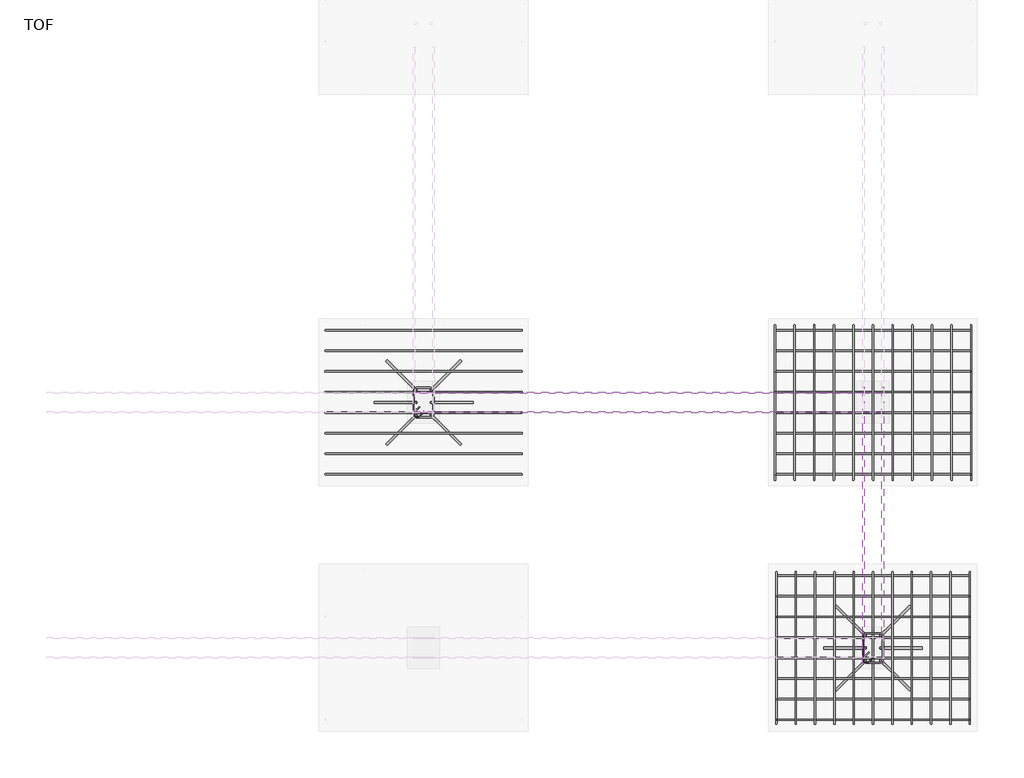
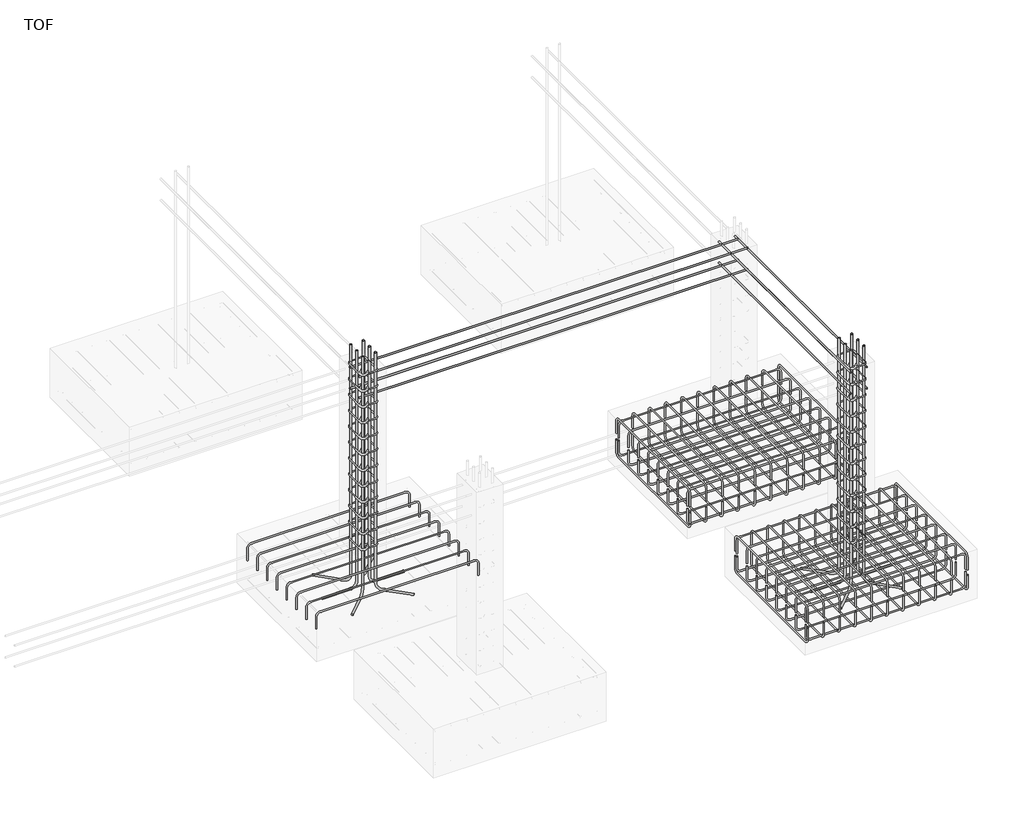
# One storey, part 7 of 10: 31 reinforcing bars.
"""IFC4 building model written with IfcOpenShell, lengths in millimetres."""

from ifc_helpers import new_model, si_unit, point, frame, origin, place, context, project, spatial, polyline, circle_curve, trimmed, segment, composite_curve, source, transform, mapped, element, save
from ifc_brep_helpers import swept_disk

model = new_model("IFC4")

# Units and contexts
model_context = context("Model", 3, world=origin())
ifc_project = project(units=[si_unit("LENGTHUNIT", "METRE", prefix="MILLI")], contexts=[model_context])

# Site, building, storey
site = spatial("IfcSite", under=ifc_project)
building = spatial("IfcBuilding", under=site)
storey = spatial("IfcBuildingStorey", under=building, Name="TOF", Elevation=-1828.8)

# Reinforcing bars
placement = place(None, origin())
reinforcing_bar_shape = source(origin(), model_context, "Body", "SolidModel", [
    swept_disk(composite_curve([segment(polyline([(13565.2782143, -14549.6267376, -2028.8), (13565.2782143, -14549.6267376, -1918.8)]), True, "CONTINUOUS"), segment(trimmed(circle_curve(frame((13565.2782143, -14584.6267376, -1918.8), z_axis=(1.0, 0.0, 0.0), x_axis=(0.0, 35.0, 0.0)), 35.0), [point((13565.2782143, -14549.6267376, -1918.8))], [point((13565.2782143, -14584.6267376, -1883.8))], True, "CARTESIAN"), True, "CONTINUOUS"), segment(polyline([(13565.2782143, -14584.6267376, -1883.8), (13565.2782143, -15604.6267376, -1883.8)]), True, "CONTINUOUS"), segment(trimmed(circle_curve(frame((13565.2782143, -15604.6267376, -1918.8), z_axis=(1.0, 0.0, 0.0), x_axis=(0.0, 0.0, 35.0)), 35.0), [point((13565.2782143, -15604.6267376, -1883.8))], [point((13565.2782143, -15639.6267376, -1918.8))], True, "CARTESIAN"), True, "CONTINUOUS"), segment(polyline([(13565.2782143, -15639.6267376, -1918.8), (13565.2782143, -15639.6267376, -2028.8)]), True, "CONTINUOUS")], self_intersect=False), 5.0),
])
element("IfcReinforcingBar", 1, at=placement, inside=storey, context=model_context, shape_type="MappedRepresentation", body=[
    mapped(reinforcing_bar_shape, transform((0.0, 0.0, 0.0), x_axis=(1.0, 0.0, 0.0), y_axis=(0.0, 1.0, 0.0), z_axis=(0.0, 0.0, 1.0))),
    mapped(reinforcing_bar_shape, transform((-139.0, 0.0, 0.0), x_axis=(1.0, 0.0, 0.0), y_axis=(0.0, 1.0, 0.0), z_axis=(0.0, 0.0, 1.0))),
    mapped(reinforcing_bar_shape, transform((-278.0, 0.0, 0.0), x_axis=(1.0, 0.0, 0.0), y_axis=(0.0, 1.0, 0.0), z_axis=(0.0, 0.0, 1.0))),
    mapped(reinforcing_bar_shape, transform((-417.0, 0.0, 0.0), x_axis=(1.0, 0.0, 0.0), y_axis=(0.0, 1.0, 0.0), z_axis=(0.0, 0.0, 1.0))),
    mapped(reinforcing_bar_shape, transform((-556.0, 0.0, 0.0), x_axis=(1.0, 0.0, 0.0), y_axis=(0.0, 1.0, 0.0), z_axis=(0.0, 0.0, 1.0))),
    mapped(reinforcing_bar_shape, transform((-695.0, 0.0, 0.0), x_axis=(1.0, 0.0, 0.0), y_axis=(0.0, 1.0, 0.0), z_axis=(0.0, 0.0, 1.0))),
    mapped(reinforcing_bar_shape, transform((-834.0, 0.0, 0.0), x_axis=(1.0, 0.0, 0.0), y_axis=(0.0, 1.0, 0.0), z_axis=(0.0, 0.0, 1.0))),
    mapped(reinforcing_bar_shape, transform((-973.0, 0.0, 0.0), x_axis=(1.0, 0.0, 0.0), y_axis=(0.0, 1.0, 0.0), z_axis=(0.0, 0.0, 1.0))),
    mapped(reinforcing_bar_shape, transform((-1112.0, 0.0, 0.0), x_axis=(1.0, 0.0, 0.0), y_axis=(0.0, 1.0, 0.0), z_axis=(0.0, 0.0, 1.0))),
    mapped(reinforcing_bar_shape, transform((-1251.0, 0.0, 0.0), x_axis=(1.0, 0.0, 0.0), y_axis=(0.0, 1.0, 0.0), z_axis=(0.0, 0.0, 1.0))),
    mapped(reinforcing_bar_shape, transform((-1390.0, 0.0, 0.0), x_axis=(1.0, 0.0, 0.0), y_axis=(0.0, 1.0, 0.0), z_axis=(0.0, 0.0, 1.0))),
])
reinforcing_bar_2_shape = source(origin(), model_context, "Body", "SolidModel", [
    swept_disk(composite_curve([segment(polyline([(13565.2782143, -15639.6267376, -2077.5233378), (13565.2782143, -15639.6267376, -2187.5233378)]), True, "CONTINUOUS"), segment(trimmed(circle_curve(frame((13565.2782143, -15604.6267376, -2187.5233378), z_axis=(1.0, 0.0, 0.0), x_axis=(0.0, -35.0, 0.0)), 35.0), [point((13565.2782143, -15639.6267376, -2187.5233378))], [point((13565.2782143, -15604.6267376, -2222.5233378))], True, "CARTESIAN"), True, "CONTINUOUS"), segment(polyline([(13565.2782143, -15604.6267376, -2222.5233378), (13565.2782143, -14584.6267376, -2222.5233378)]), True, "CONTINUOUS"), segment(trimmed(circle_curve(frame((13565.2782143, -14584.6267376, -2187.5233378), z_axis=(1.0, 0.0, 0.0), x_axis=(0.0, 0.0, -35.0)), 35.0), [point((13565.2782143, -14584.6267376, -2222.5233378))], [point((13565.2782143, -14549.6267376, -2187.5233378))], True, "CARTESIAN"), True, "CONTINUOUS"), segment(polyline([(13565.2782143, -14549.6267376, -2187.5233378), (13565.2782143, -14549.6267376, -2077.5233378)]), True, "CONTINUOUS")], self_intersect=False), 5.0),
])
element("IfcReinforcingBar", 2, at=placement, inside=storey, context=model_context, shape_type="MappedRepresentation", body=[
    mapped(reinforcing_bar_2_shape, transform((0.0, 0.0, 0.0), x_axis=(1.0, 0.0, 0.0), y_axis=(0.0, 1.0, 0.0), z_axis=(0.0, 0.0, 1.0))),
    mapped(reinforcing_bar_2_shape, transform((-139.0, 0.0, 0.0), x_axis=(1.0, 0.0, 0.0), y_axis=(0.0, 1.0, 0.0), z_axis=(0.0, 0.0, 1.0))),
    mapped(reinforcing_bar_2_shape, transform((-278.0, 0.0, 0.0), x_axis=(1.0, 0.0, 0.0), y_axis=(0.0, 1.0, 0.0), z_axis=(0.0, 0.0, 1.0))),
    mapped(reinforcing_bar_2_shape, transform((-417.0, 0.0, 0.0), x_axis=(1.0, 0.0, 0.0), y_axis=(0.0, 1.0, 0.0), z_axis=(0.0, 0.0, 1.0))),
    mapped(reinforcing_bar_2_shape, transform((-556.0, 0.0, 0.0), x_axis=(1.0, 0.0, 0.0), y_axis=(0.0, 1.0, 0.0), z_axis=(0.0, 0.0, 1.0))),
    mapped(reinforcing_bar_2_shape, transform((-695.0, 0.0, 0.0), x_axis=(1.0, 0.0, 0.0), y_axis=(0.0, 1.0, 0.0), z_axis=(0.0, 0.0, 1.0))),
    mapped(reinforcing_bar_2_shape, transform((-834.0, 0.0, 0.0), x_axis=(1.0, 0.0, 0.0), y_axis=(0.0, 1.0, 0.0), z_axis=(0.0, 0.0, 1.0))),
    mapped(reinforcing_bar_2_shape, transform((-973.0, 0.0, 0.0), x_axis=(1.0, 0.0, 0.0), y_axis=(0.0, 1.0, 0.0), z_axis=(0.0, 0.0, 1.0))),
    mapped(reinforcing_bar_2_shape, transform((-1112.0, 0.0, 0.0), x_axis=(1.0, 0.0, 0.0), y_axis=(0.0, 1.0, 0.0), z_axis=(0.0, 0.0, 1.0))),
    mapped(reinforcing_bar_2_shape, transform((-1251.0, 0.0, 0.0), x_axis=(1.0, 0.0, 0.0), y_axis=(0.0, 1.0, 0.0), z_axis=(0.0, 0.0, 1.0))),
    mapped(reinforcing_bar_2_shape, transform((-1390.0, 0.0, 0.0), x_axis=(1.0, 0.0, 0.0), y_axis=(0.0, 1.0, 0.0), z_axis=(0.0, 0.0, 1.0))),
])
reinforcing_bar_3_shape = source(origin(), model_context, "Body", "SolidModel", [
    swept_disk(composite_curve([segment(polyline([(13565.2782143, -14574.6861459, -2066.1776706), (13565.2782143, -14574.6861459, -2176.1776706)]), True, "CONTINUOUS"), segment(trimmed(circle_curve(frame((13530.2782143, -14574.6861459, -2176.1776706), z_axis=(0.0, 1.0, 0.0), x_axis=(35.0, 0.0, 0.0)), 35.0), [point((13565.2782143, -14574.6861459, -2176.1776706))], [point((13530.2782143, -14574.6861459, -2211.1776706))], True, "CARTESIAN"), True, "CONTINUOUS"), segment(polyline([(13530.2782143, -14574.6861459, -2211.1776706), (12210.2782143, -14574.6861459, -2211.1776706)]), True, "CONTINUOUS"), segment(trimmed(circle_curve(frame((12210.2782143, -14574.6861459, -2176.1776706), z_axis=(0.0, 1.0, 0.0), x_axis=(0.0, 0.0, -35.0)), 35.0), [point((12210.2782143, -14574.6861459, -2211.1776706))], [point((12175.2782143, -14574.6861459, -2176.1776706))], True, "CARTESIAN"), True, "CONTINUOUS"), segment(polyline([(12175.2782143, -14574.6861459, -2176.1776706), (12175.2782143, -14574.6861459, -2066.1776706)]), True, "CONTINUOUS")], self_intersect=False), 5.0),
])
element("IfcReinforcingBar", 3, at=placement, inside=storey, context=model_context, shape_type="MappedRepresentation", body=[
    mapped(reinforcing_bar_3_shape, transform((0.0, 0.0, 0.0), x_axis=(1.0, 0.0, 0.0), y_axis=(0.0, 1.0, 0.0), z_axis=(0.0, 0.0, 1.0))),
    mapped(reinforcing_bar_3_shape, transform((0.0, -148.0321606, 0.0), x_axis=(1.0, 0.0, 0.0), y_axis=(0.0, 1.0, 0.0), z_axis=(0.0, 0.0, 1.0))),
    mapped(reinforcing_bar_3_shape, transform((0.0, -296.0643211, 0.0), x_axis=(1.0, 0.0, 0.0), y_axis=(0.0, 1.0, 0.0), z_axis=(0.0, 0.0, 1.0))),
    mapped(reinforcing_bar_3_shape, transform((0.0, -444.0964817, 0.0), x_axis=(1.0, 0.0, 0.0), y_axis=(0.0, 1.0, 0.0), z_axis=(0.0, 0.0, 1.0))),
    mapped(reinforcing_bar_3_shape, transform((0.0, -592.1286423, 0.0), x_axis=(1.0, 0.0, 0.0), y_axis=(0.0, 1.0, 0.0), z_axis=(0.0, 0.0, 1.0))),
    mapped(reinforcing_bar_3_shape, transform((0.0, -740.1608029, 0.0), x_axis=(1.0, 0.0, 0.0), y_axis=(0.0, 1.0, 0.0), z_axis=(0.0, 0.0, 1.0))),
    mapped(reinforcing_bar_3_shape, transform((0.0, -888.1929634, 0.0), x_axis=(1.0, 0.0, 0.0), y_axis=(0.0, 1.0, 0.0), z_axis=(0.0, 0.0, 1.0))),
    mapped(reinforcing_bar_3_shape, transform((0.0, -1036.225124, 0.0), x_axis=(1.0, 0.0, 0.0), y_axis=(0.0, 1.0, 0.0), z_axis=(0.0, 0.0, 1.0))),
])
reinforcing_bar_4_shape = source(origin(), model_context, "Body", "SolidModel", [
    swept_disk(composite_curve([segment(polyline([(13565.2782143, -15610.9112699, -2039.256778), (13565.2782143, -15610.9112699, -1929.256778)]), True, "CONTINUOUS"), segment(trimmed(circle_curve(frame((13530.2782143, -15610.9112699, -1929.256778), z_axis=(0.0, -1.0, 0.0), x_axis=(35.0, 0.0, 0.0)), 35.0), [point((13565.2782143, -15610.9112699, -1929.256778))], [point((13530.2782143, -15610.9112699, -1894.256778))], True, "CARTESIAN"), True, "CONTINUOUS"), segment(polyline([(13530.2782143, -15610.9112699, -1894.256778), (12210.2782143, -15610.9112699, -1894.256778)]), True, "CONTINUOUS"), segment(trimmed(circle_curve(frame((12210.2782143, -15610.9112699, -1929.256778), z_axis=(0.0, -1.0, 0.0), x_axis=(0.0, 0.0, 35.0)), 35.0), [point((12210.2782143, -15610.9112699, -1894.256778))], [point((12175.2782143, -15610.9112699, -1929.256778))], True, "CARTESIAN"), True, "CONTINUOUS"), segment(polyline([(12175.2782143, -15610.9112699, -1929.256778), (12175.2782143, -15610.9112699, -2039.256778)]), True, "CONTINUOUS")], self_intersect=False), 5.0),
])
element("IfcReinforcingBar", 4, at=placement, inside=storey, context=model_context, shape_type="MappedRepresentation", body=[
    mapped(reinforcing_bar_4_shape, transform((0.0, 0.0, 0.0), x_axis=(1.0, 0.0, 0.0), y_axis=(0.0, 1.0, 0.0), z_axis=(0.0, 0.0, 1.0))),
    mapped(reinforcing_bar_4_shape, transform((0.0, 148.0321606, 0.0), x_axis=(1.0, 0.0, 0.0), y_axis=(0.0, 1.0, 0.0), z_axis=(0.0, 0.0, 1.0))),
    mapped(reinforcing_bar_4_shape, transform((0.0, 296.0643211, 0.0), x_axis=(1.0, 0.0, 0.0), y_axis=(0.0, 1.0, 0.0), z_axis=(0.0, 0.0, 1.0))),
    mapped(reinforcing_bar_4_shape, transform((0.0, 444.0964817, 0.0), x_axis=(1.0, 0.0, 0.0), y_axis=(0.0, 1.0, 0.0), z_axis=(0.0, 0.0, 1.0))),
    mapped(reinforcing_bar_4_shape, transform((0.0, 592.1286423, 0.0), x_axis=(1.0, 0.0, 0.0), y_axis=(0.0, 1.0, 0.0), z_axis=(0.0, 0.0, 1.0))),
    mapped(reinforcing_bar_4_shape, transform((0.0, 740.1608029, 0.0), x_axis=(1.0, 0.0, 0.0), y_axis=(0.0, 1.0, 0.0), z_axis=(0.0, 0.0, 1.0))),
    mapped(reinforcing_bar_4_shape, transform((0.0, 888.1929634, 0.0), x_axis=(1.0, 0.0, 0.0), y_axis=(0.0, 1.0, 0.0), z_axis=(0.0, 0.0, 1.0))),
    mapped(reinforcing_bar_4_shape, transform((0.0, 1036.225124, 0.0), x_axis=(1.0, 0.0, 0.0), y_axis=(0.0, 1.0, 0.0), z_axis=(0.0, 0.0, 1.0))),
])
reinforcing_bar_5_shape = source(origin(), model_context, "Body", "SolidModel", [
    swept_disk(composite_curve([segment(polyline([(10345.2782143, -13845.9112699, -2039.256778), (10345.2782143, -13845.9112699, -1929.256778)]), True, "CONTINUOUS"), segment(trimmed(circle_curve(frame((10310.2782143, -13845.9112699, -1929.256778), z_axis=(0.0, -1.0, 0.0), x_axis=(35.0, 0.0, 0.0)), 35.0), [point((10345.2782143, -13845.9112699, -1929.256778))], [point((10310.2782143, -13845.9112699, -1894.256778))], True, "CARTESIAN"), True, "CONTINUOUS"), segment(polyline([(10310.2782143, -13845.9112699, -1894.256778), (8970.2782143, -13845.9112699, -1894.256778)]), True, "CONTINUOUS"), segment(trimmed(circle_curve(frame((8970.2782143, -13845.9112699, -1929.256778), z_axis=(0.0, -1.0, 0.0), x_axis=(0.0, 0.0, 35.0)), 35.0), [point((8970.2782143, -13845.9112699, -1894.256778))], [point((8935.2782143, -13845.9112699, -1929.256778))], True, "CARTESIAN"), True, "CONTINUOUS"), segment(polyline([(8935.2782143, -13845.9112699, -1929.256778), (8935.2782143, -13845.9112699, -2039.256778)]), True, "CONTINUOUS")], self_intersect=False), 5.0),
])
element("IfcReinforcingBar", 5, at=placement, inside=storey, context=model_context, shape_type="MappedRepresentation", body=[
    mapped(reinforcing_bar_5_shape, transform((0.0, 0.0, 0.0), x_axis=(1.0, 0.0, 0.0), y_axis=(0.0, 1.0, 0.0), z_axis=(0.0, 0.0, 1.0))),
    mapped(reinforcing_bar_5_shape, transform((0.0, 148.0321606, 0.0), x_axis=(1.0, 0.0, 0.0), y_axis=(0.0, 1.0, 0.0), z_axis=(0.0, 0.0, 1.0))),
    mapped(reinforcing_bar_5_shape, transform((0.0, 296.0643211, 0.0), x_axis=(1.0, 0.0, 0.0), y_axis=(0.0, 1.0, 0.0), z_axis=(0.0, 0.0, 1.0))),
    mapped(reinforcing_bar_5_shape, transform((0.0, 444.0964817, 0.0), x_axis=(1.0, 0.0, 0.0), y_axis=(0.0, 1.0, 0.0), z_axis=(0.0, 0.0, 1.0))),
    mapped(reinforcing_bar_5_shape, transform((0.0, 592.1286423, 0.0), x_axis=(1.0, 0.0, 0.0), y_axis=(0.0, 1.0, 0.0), z_axis=(0.0, 0.0, 1.0))),
    mapped(reinforcing_bar_5_shape, transform((0.0, 740.1608029, 0.0), x_axis=(1.0, 0.0, 0.0), y_axis=(0.0, 1.0, 0.0), z_axis=(0.0, 0.0, 1.0))),
    mapped(reinforcing_bar_5_shape, transform((0.0, 888.1929634, 0.0), x_axis=(1.0, 0.0, 0.0), y_axis=(0.0, 1.0, 0.0), z_axis=(0.0, 0.0, 1.0))),
    mapped(reinforcing_bar_5_shape, transform((0.0, 1036.225124, 0.0), x_axis=(1.0, 0.0, 0.0), y_axis=(0.0, 1.0, 0.0), z_axis=(0.0, 0.0, 1.0))),
])
reinforcing_bar_6_shape = source(origin(), model_context, "Body", "SolidModel", [
    swept_disk(composite_curve([segment(polyline([(13575.2782143, -12774.6267376, -2018.8), (13575.2782143, -12774.6267376, -1908.8)]), True, "CONTINUOUS"), segment(trimmed(circle_curve(frame((13575.2782143, -12809.6267376, -1908.8), z_axis=(1.0, 0.0, 0.0), x_axis=(0.0, 35.0, 0.0)), 35.0), [point((13575.2782143, -12774.6267376, -1908.8))], [point((13575.2782143, -12809.6267376, -1873.8))], True, "CARTESIAN"), True, "CONTINUOUS"), segment(polyline([(13575.2782143, -12809.6267376, -1873.8), (13575.2782143, -13849.6267376, -1873.8)]), True, "CONTINUOUS"), segment(trimmed(circle_curve(frame((13575.2782143, -13849.6267376, -1908.8), z_axis=(1.0, 0.0, 0.0), x_axis=(0.0, 0.0, 35.0)), 35.0), [point((13575.2782143, -13849.6267376, -1873.8))], [point((13575.2782143, -13884.6267376, -1908.8))], True, "CARTESIAN"), True, "CONTINUOUS"), segment(polyline([(13575.2782143, -13884.6267376, -1908.8), (13575.2782143, -13884.6267376, -2018.8)]), True, "CONTINUOUS")], self_intersect=False), 5.0),
])
element("IfcReinforcingBar", 6, at=placement, inside=storey, context=model_context, shape_type="MappedRepresentation", body=[
    mapped(reinforcing_bar_6_shape, transform((0.0, 0.0, 0.0), x_axis=(1.0, 0.0, 0.0), y_axis=(0.0, 1.0, 0.0), z_axis=(0.0, 0.0, 1.0))),
    mapped(reinforcing_bar_6_shape, transform((-141.0, 0.0, 0.0), x_axis=(1.0, 0.0, 0.0), y_axis=(0.0, 1.0, 0.0), z_axis=(0.0, 0.0, 1.0))),
    mapped(reinforcing_bar_6_shape, transform((-282.0, 0.0, 0.0), x_axis=(1.0, 0.0, 0.0), y_axis=(0.0, 1.0, 0.0), z_axis=(0.0, 0.0, 1.0))),
    mapped(reinforcing_bar_6_shape, transform((-423.0, 0.0, 0.0), x_axis=(1.0, 0.0, 0.0), y_axis=(0.0, 1.0, 0.0), z_axis=(0.0, 0.0, 1.0))),
    mapped(reinforcing_bar_6_shape, transform((-564.0, 0.0, 0.0), x_axis=(1.0, 0.0, 0.0), y_axis=(0.0, 1.0, 0.0), z_axis=(0.0, 0.0, 1.0))),
    mapped(reinforcing_bar_6_shape, transform((-705.0, 0.0, 0.0), x_axis=(1.0, 0.0, 0.0), y_axis=(0.0, 1.0, 0.0), z_axis=(0.0, 0.0, 1.0))),
    mapped(reinforcing_bar_6_shape, transform((-846.0, 0.0, 0.0), x_axis=(1.0, 0.0, 0.0), y_axis=(0.0, 1.0, 0.0), z_axis=(0.0, 0.0, 1.0))),
    mapped(reinforcing_bar_6_shape, transform((-987.0, 0.0, 0.0), x_axis=(1.0, 0.0, 0.0), y_axis=(0.0, 1.0, 0.0), z_axis=(0.0, 0.0, 1.0))),
    mapped(reinforcing_bar_6_shape, transform((-1128.0, 0.0, 0.0), x_axis=(1.0, 0.0, 0.0), y_axis=(0.0, 1.0, 0.0), z_axis=(0.0, 0.0, 1.0))),
    mapped(reinforcing_bar_6_shape, transform((-1269.0, 0.0, 0.0), x_axis=(1.0, 0.0, 0.0), y_axis=(0.0, 1.0, 0.0), z_axis=(0.0, 0.0, 1.0))),
    mapped(reinforcing_bar_6_shape, transform((-1410.0, 0.0, 0.0), x_axis=(1.0, 0.0, 0.0), y_axis=(0.0, 1.0, 0.0), z_axis=(0.0, 0.0, 1.0))),
])
reinforcing_bar_7_shape = source(origin(), model_context, "Body", "SolidModel", [
    swept_disk(composite_curve([segment(polyline([(13575.2782143, -13884.6267376, -2077.5233378), (13575.2782143, -13884.6267376, -2187.5233378)]), True, "CONTINUOUS"), segment(trimmed(circle_curve(frame((13575.2782143, -13849.6267376, -2187.5233378), z_axis=(1.0, 0.0, 0.0), x_axis=(0.0, -35.0, 0.0)), 35.0), [point((13575.2782143, -13884.6267376, -2187.5233378))], [point((13575.2782143, -13849.6267376, -2222.5233378))], True, "CARTESIAN"), True, "CONTINUOUS"), segment(polyline([(13575.2782143, -13849.6267376, -2222.5233378), (13575.2782143, -12809.6267376, -2222.5233378)]), True, "CONTINUOUS"), segment(trimmed(circle_curve(frame((13575.2782143, -12809.6267376, -2187.5233378), z_axis=(1.0, 0.0, 0.0), x_axis=(0.0, 0.0, -35.0)), 35.0), [point((13575.2782143, -12809.6267376, -2222.5233378))], [point((13575.2782143, -12774.6267376, -2187.5233378))], True, "CARTESIAN"), True, "CONTINUOUS"), segment(polyline([(13575.2782143, -12774.6267376, -2187.5233378), (13575.2782143, -12774.6267376, -2077.5233378)]), True, "CONTINUOUS")], self_intersect=False), 5.0),
])
element("IfcReinforcingBar", 7, at=placement, inside=storey, context=model_context, shape_type="MappedRepresentation", body=[
    mapped(reinforcing_bar_7_shape, transform((0.0, 0.0, 0.0), x_axis=(1.0, 0.0, 0.0), y_axis=(0.0, 1.0, 0.0), z_axis=(0.0, 0.0, 1.0))),
    mapped(reinforcing_bar_7_shape, transform((-141.0, 0.0, 0.0), x_axis=(1.0, 0.0, 0.0), y_axis=(0.0, 1.0, 0.0), z_axis=(0.0, 0.0, 1.0))),
    mapped(reinforcing_bar_7_shape, transform((-282.0, 0.0, 0.0), x_axis=(1.0, 0.0, 0.0), y_axis=(0.0, 1.0, 0.0), z_axis=(0.0, 0.0, 1.0))),
    mapped(reinforcing_bar_7_shape, transform((-423.0, 0.0, 0.0), x_axis=(1.0, 0.0, 0.0), y_axis=(0.0, 1.0, 0.0), z_axis=(0.0, 0.0, 1.0))),
    mapped(reinforcing_bar_7_shape, transform((-564.0, 0.0, 0.0), x_axis=(1.0, 0.0, 0.0), y_axis=(0.0, 1.0, 0.0), z_axis=(0.0, 0.0, 1.0))),
    mapped(reinforcing_bar_7_shape, transform((-705.0, 0.0, 0.0), x_axis=(1.0, 0.0, 0.0), y_axis=(0.0, 1.0, 0.0), z_axis=(0.0, 0.0, 1.0))),
    mapped(reinforcing_bar_7_shape, transform((-846.0, 0.0, 0.0), x_axis=(1.0, 0.0, 0.0), y_axis=(0.0, 1.0, 0.0), z_axis=(0.0, 0.0, 1.0))),
    mapped(reinforcing_bar_7_shape, transform((-987.0, 0.0, 0.0), x_axis=(1.0, 0.0, 0.0), y_axis=(0.0, 1.0, 0.0), z_axis=(0.0, 0.0, 1.0))),
    mapped(reinforcing_bar_7_shape, transform((-1128.0, 0.0, 0.0), x_axis=(1.0, 0.0, 0.0), y_axis=(0.0, 1.0, 0.0), z_axis=(0.0, 0.0, 1.0))),
    mapped(reinforcing_bar_7_shape, transform((-1269.0, 0.0, 0.0), x_axis=(1.0, 0.0, 0.0), y_axis=(0.0, 1.0, 0.0), z_axis=(0.0, 0.0, 1.0))),
    mapped(reinforcing_bar_7_shape, transform((-1410.0, 0.0, 0.0), x_axis=(1.0, 0.0, 0.0), y_axis=(0.0, 1.0, 0.0), z_axis=(0.0, 0.0, 1.0))),
])
reinforcing_bar_8_shape = source(origin(), model_context, "Body", "SolidModel", [
    swept_disk(composite_curve([segment(polyline([(13575.2782143, -12809.6861459, -2066.1776706), (13575.2782143, -12809.6861459, -2176.1776706)]), True, "CONTINUOUS"), segment(trimmed(circle_curve(frame((13540.2782143, -12809.6861459, -2176.1776706), z_axis=(0.0, 1.0, 0.0), x_axis=(35.0, 0.0, 0.0)), 35.0), [point((13575.2782143, -12809.6861459, -2176.1776706))], [point((13540.2782143, -12809.6861459, -2211.1776706))], True, "CARTESIAN"), True, "CONTINUOUS"), segment(polyline([(13540.2782143, -12809.6861459, -2211.1776706), (12200.2782143, -12809.6861459, -2211.1776706)]), True, "CONTINUOUS"), segment(trimmed(circle_curve(frame((12200.2782143, -12809.6861459, -2176.1776706), z_axis=(0.0, 1.0, 0.0), x_axis=(0.0, 0.0, -35.0)), 35.0), [point((12200.2782143, -12809.6861459, -2211.1776706))], [point((12165.2782143, -12809.6861459, -2176.1776706))], True, "CARTESIAN"), True, "CONTINUOUS"), segment(polyline([(12165.2782143, -12809.6861459, -2176.1776706), (12165.2782143, -12809.6861459, -2066.1776706)]), True, "CONTINUOUS")], self_intersect=False), 5.0),
])
element("IfcReinforcingBar", 8, at=placement, inside=storey, context=model_context, shape_type="MappedRepresentation", body=[
    mapped(reinforcing_bar_8_shape, transform((0.0, 0.0, 0.0), x_axis=(1.0, 0.0, 0.0), y_axis=(0.0, 1.0, 0.0), z_axis=(0.0, 0.0, 1.0))),
    mapped(reinforcing_bar_8_shape, transform((0.0, -148.0321606, 0.0), x_axis=(1.0, 0.0, 0.0), y_axis=(0.0, 1.0, 0.0), z_axis=(0.0, 0.0, 1.0))),
    mapped(reinforcing_bar_8_shape, transform((0.0, -296.0643211, 0.0), x_axis=(1.0, 0.0, 0.0), y_axis=(0.0, 1.0, 0.0), z_axis=(0.0, 0.0, 1.0))),
    mapped(reinforcing_bar_8_shape, transform((0.0, -444.0964817, 0.0), x_axis=(1.0, 0.0, 0.0), y_axis=(0.0, 1.0, 0.0), z_axis=(0.0, 0.0, 1.0))),
    mapped(reinforcing_bar_8_shape, transform((0.0, -592.1286423, 0.0), x_axis=(1.0, 0.0, 0.0), y_axis=(0.0, 1.0, 0.0), z_axis=(0.0, 0.0, 1.0))),
    mapped(reinforcing_bar_8_shape, transform((0.0, -740.1608029, 0.0), x_axis=(1.0, 0.0, 0.0), y_axis=(0.0, 1.0, 0.0), z_axis=(0.0, 0.0, 1.0))),
    mapped(reinforcing_bar_8_shape, transform((0.0, -888.1929634, 0.0), x_axis=(1.0, 0.0, 0.0), y_axis=(0.0, 1.0, 0.0), z_axis=(0.0, 0.0, 1.0))),
    mapped(reinforcing_bar_8_shape, transform((0.0, -1036.225124, 0.0), x_axis=(1.0, 0.0, 0.0), y_axis=(0.0, 1.0, 0.0), z_axis=(0.0, 0.0, 1.0))),
])
reinforcing_bar_9_shape = source(origin(), model_context, "Body", "SolidModel", [
    swept_disk(composite_curve([segment(polyline([(13575.2782143, -13845.9112699, -2039.256778), (13575.2782143, -13845.9112699, -1929.256778)]), True, "CONTINUOUS"), segment(trimmed(circle_curve(frame((13540.2782143, -13845.9112699, -1929.256778), z_axis=(0.0, -1.0, 0.0), x_axis=(35.0, 0.0, 0.0)), 35.0), [point((13575.2782143, -13845.9112699, -1929.256778))], [point((13540.2782143, -13845.9112699, -1894.256778))], True, "CARTESIAN"), True, "CONTINUOUS"), segment(polyline([(13540.2782143, -13845.9112699, -1894.256778), (12200.2782143, -13845.9112699, -1894.256778)]), True, "CONTINUOUS"), segment(trimmed(circle_curve(frame((12200.2782143, -13845.9112699, -1929.256778), z_axis=(0.0, -1.0, 0.0), x_axis=(0.0, 0.0, 35.0)), 35.0), [point((12200.2782143, -13845.9112699, -1894.256778))], [point((12165.2782143, -13845.9112699, -1929.256778))], True, "CARTESIAN"), True, "CONTINUOUS"), segment(polyline([(12165.2782143, -13845.9112699, -1929.256778), (12165.2782143, -13845.9112699, -2039.256778)]), True, "CONTINUOUS")], self_intersect=False), 5.0),
])
element("IfcReinforcingBar", 9, at=placement, inside=storey, context=model_context, shape_type="MappedRepresentation", body=[
    mapped(reinforcing_bar_9_shape, transform((0.0, 0.0, 0.0), x_axis=(1.0, 0.0, 0.0), y_axis=(0.0, 1.0, 0.0), z_axis=(0.0, 0.0, 1.0))),
    mapped(reinforcing_bar_9_shape, transform((0.0, 148.0321606, 0.0), x_axis=(1.0, 0.0, 0.0), y_axis=(0.0, 1.0, 0.0), z_axis=(0.0, 0.0, 1.0))),
    mapped(reinforcing_bar_9_shape, transform((0.0, 296.0643211, 0.0), x_axis=(1.0, 0.0, 0.0), y_axis=(0.0, 1.0, 0.0), z_axis=(0.0, 0.0, 1.0))),
    mapped(reinforcing_bar_9_shape, transform((0.0, 444.0964817, 0.0), x_axis=(1.0, 0.0, 0.0), y_axis=(0.0, 1.0, 0.0), z_axis=(0.0, 0.0, 1.0))),
    mapped(reinforcing_bar_9_shape, transform((0.0, 592.1286423, 0.0), x_axis=(1.0, 0.0, 0.0), y_axis=(0.0, 1.0, 0.0), z_axis=(0.0, 0.0, 1.0))),
    mapped(reinforcing_bar_9_shape, transform((0.0, 740.1608029, 0.0), x_axis=(1.0, 0.0, 0.0), y_axis=(0.0, 1.0, 0.0), z_axis=(0.0, 0.0, 1.0))),
    mapped(reinforcing_bar_9_shape, transform((0.0, 888.1929634, 0.0), x_axis=(1.0, 0.0, 0.0), y_axis=(0.0, 1.0, 0.0), z_axis=(0.0, 0.0, 1.0))),
    mapped(reinforcing_bar_9_shape, transform((0.0, 1036.225124, 0.0), x_axis=(1.0, 0.0, 0.0), y_axis=(0.0, 1.0, 0.0), z_axis=(0.0, 0.0, 1.0))),
])
reinforcing_bar_10_shape = source(origin(), model_context, "Body", "SolidModel", [
    swept_disk(composite_curve([segment(polyline([(12840.248777, -15125.7150493, -1784.8), (12806.3076515, -15159.6561748, -1784.8)]), True, "CONTINUOUS"), segment(trimmed(circle_curve(frame((12823.2782143, -15176.6267376, -1784.8), z_axis=(0.0, 0.0, 1.0), x_axis=(-16.970562800001062, 16.970562799999243, 0.0)), 24.0), [point((12806.3076515, -15159.6561748, -1784.8))], [point((12823.2782143, -15200.6267376, -1784.8))], True, "CARTESIAN"), True, "CONTINUOUS"), segment(polyline([(12823.2782143, -15200.6267376, -1784.8), (12917.2782143, -15200.6267376, -1784.8)]), True, "CONTINUOUS"), segment(trimmed(circle_curve(frame((12917.2782143, -15176.6267376, -1784.8), z_axis=(0.0, 0.0, 1.0), x_axis=(0.0, -24.0, 0.0)), 24.0), [point((12917.2782143, -15200.6267376, -1784.8))], [point((12941.2782143, -15176.6267376, -1784.8))], True, "CARTESIAN"), True, "CONTINUOUS"), segment(polyline([(12941.2782143, -15176.6267376, -1784.8), (12941.2782143, -15012.6267376, -1784.8)]), True, "CONTINUOUS"), segment(trimmed(circle_curve(frame((12917.3162115, -15012.6267376, -1786.149972), z_axis=(-0.05624883273897078, 0.0, 0.9984167811167355), x_axis=(23.962002800000846, 0.0, 1.3499719999999797)), 24.0), [point((12941.2782143, -15012.6267376, -1784.8))], [point((12917.3162115, -14988.6267376, -1786.149972))], True, "CARTESIAN"), True, "CONTINUOUS"), segment(polyline([(12917.3162115, -14988.6267376, -1786.149972), (12823.240217, -14988.6267376, -1791.450028)]), True, "CONTINUOUS"), segment(trimmed(circle_curve(frame((12823.240217, -15012.6267376, -1791.450028), z_axis=(-0.05624883273897078, 0.0, 0.9984167811167355), x_axis=(0.0, 24.0, 0.0)), 24.0), [point((12823.240217, -14988.6267376, -1791.450028))], [point((12799.2782143, -15012.6267376, -1792.8))], True, "CARTESIAN"), True, "CONTINUOUS"), segment(polyline([(12799.2782143, -15012.6267376, -1792.8), (12799.2782143, -15176.6267376, -1792.8)]), True, "CONTINUOUS"), segment(trimmed(circle_curve(frame((12823.2782143, -15176.6267376, -1792.8), z_axis=(0.0, 0.0, 1.0), x_axis=(-24.0, 0.0, 0.0)), 24.0), [point((12799.2782143, -15176.6267376, -1792.8))], [point((12840.248777, -15193.5973003, -1792.8))], True, "CARTESIAN"), True, "CONTINUOUS"), segment(polyline([(12840.248777, -15193.5973003, -1792.8), (12874.1899025, -15159.6561748, -1792.8)]), True, "CONTINUOUS")], self_intersect=False), 4.0),
])
element("IfcReinforcingBar", 10, at=placement, inside=storey, context=model_context, shape_type="MappedRepresentation", body=[
    mapped(reinforcing_bar_10_shape, transform((0.0, 0.0, 0.0), x_axis=(1.0, 0.0, 0.0), y_axis=(0.0, 1.0, 0.0), z_axis=(0.0, 0.0, 1.0))),
    mapped(reinforcing_bar_10_shape, transform((0.0, 0.0, 145.9395608), x_axis=(1.0, 0.0, 0.0), y_axis=(0.0, 1.0, 0.0), z_axis=(0.0, 0.0, 1.0))),
    mapped(reinforcing_bar_10_shape, transform((0.0, 0.0, 291.8791216), x_axis=(1.0, 0.0, 0.0), y_axis=(0.0, 1.0, 0.0), z_axis=(0.0, 0.0, 1.0))),
    mapped(reinforcing_bar_10_shape, transform((0.0, 0.0, 437.8186825), x_axis=(1.0, 0.0, 0.0), y_axis=(0.0, 1.0, 0.0), z_axis=(0.0, 0.0, 1.0))),
    mapped(reinforcing_bar_10_shape, transform((0.0, 0.0, 583.7582433), x_axis=(1.0, 0.0, 0.0), y_axis=(0.0, 1.0, 0.0), z_axis=(0.0, 0.0, 1.0))),
    mapped(reinforcing_bar_10_shape, transform((0.0, 0.0, 729.6978041), x_axis=(1.0, 0.0, 0.0), y_axis=(0.0, 1.0, 0.0), z_axis=(0.0, 0.0, 1.0))),
    mapped(reinforcing_bar_10_shape, transform((0.0, 0.0, 875.6373649), x_axis=(1.0, 0.0, 0.0), y_axis=(0.0, 1.0, 0.0), z_axis=(0.0, 0.0, 1.0))),
    mapped(reinforcing_bar_10_shape, transform((0.0, 0.0, 1021.5769258), x_axis=(1.0, 0.0, 0.0), y_axis=(0.0, 1.0, 0.0), z_axis=(0.0, 0.0, 1.0))),
    mapped(reinforcing_bar_10_shape, transform((0.0, 0.0, 1167.5164866), x_axis=(1.0, 0.0, 0.0), y_axis=(0.0, 1.0, 0.0), z_axis=(0.0, 0.0, 1.0))),
    mapped(reinforcing_bar_10_shape, transform((0.0, 0.0, 1313.4560474), x_axis=(1.0, 0.0, 0.0), y_axis=(0.0, 1.0, 0.0), z_axis=(0.0, 0.0, 1.0))),
    mapped(reinforcing_bar_10_shape, transform((0.0, 0.0, 1459.3956082), x_axis=(1.0, 0.0, 0.0), y_axis=(0.0, 1.0, 0.0), z_axis=(0.0, 0.0, 1.0))),
    mapped(reinforcing_bar_10_shape, transform((0.0, 0.0, 1605.3351691), x_axis=(1.0, 0.0, 0.0), y_axis=(0.0, 1.0, 0.0), z_axis=(0.0, 0.0, 1.0))),
])
element("IfcReinforcingBar", 11, at=placement, inside=storey, context=model_context, shape_type="SolidModel", body=[
    swept_disk(composite_curve([segment(polyline([(12925.884816, -15185.2333393, -20.0), (12925.884816, -15185.2333393, -2138.7824747)]), True, "CONTINUOUS"), segment(trimmed(circle_curve(frame((12965.1292424, -15224.4777657, -2138.7824747), z_axis=(-0.7071067811865545, -0.7071067811865406, 0.0), x_axis=(-39.24442640000052, 39.2444263999987, 0.0)), 55.5), [point((12925.884816, -15185.2333393, -2138.7824747))], [point((12965.1292424, -15224.4777657, -2194.2824747))], True, "CARTESIAN"), True, "CONTINUOUS"), segment(polyline([(12965.1292424, -15224.4777657, -2194.2824747), (13137.5083915, -15396.8569148, -2194.2824747)]), True, "CONTINUOUS")], self_intersect=False), 8.0),
])
element("IfcReinforcingBar", 12, at=placement, inside=storey, context=model_context, shape_type="SolidModel", body=[
    swept_disk(composite_curve([segment(polyline([(12925.934816, -15094.6267376, -20.0), (12925.934816, -15094.6267376, -2138.7824747)]), True, "CONTINUOUS"), segment(trimmed(circle_curve(frame((12981.434816, -15094.6267376, -2138.7824747), z_axis=(0.0, -1.0, 0.0), x_axis=(-55.5, 0.0, 0.0)), 55.5), [point((12925.934816, -15094.6267376, -2138.7824747))], [point((12981.434816, -15094.6267376, -2194.2824747))], True, "CARTESIAN"), True, "CONTINUOUS"), segment(polyline([(12981.434816, -15094.6267376, -2194.2824747), (13225.1657466, -15094.6267376, -2194.2824747)]), True, "CONTINUOUS")], self_intersect=False), 8.0),
])
element("IfcReinforcingBar", 13, at=placement, inside=storey, context=model_context, shape_type="SolidModel", body=[
    swept_disk(composite_curve([segment(polyline([(12925.884816, -15004.0201359, -20.0), (12925.884816, -15004.0201359, -2138.7824747)]), True, "CONTINUOUS"), segment(trimmed(circle_curve(frame((12965.1292424, -14964.7757095, -2138.7824747), z_axis=(0.7071067811865545, -0.7071067811865407, 0.0), x_axis=(-39.24442640000052, -39.24442640000052, 0.0)), 55.5), [point((12925.884816, -15004.0201359, -2138.7824747))], [point((12965.1292424, -14964.7757095, -2194.2824747))], True, "CARTESIAN"), True, "CONTINUOUS"), segment(polyline([(12965.1292424, -14964.7757095, -2194.2824747), (13137.5083915, -14792.3965603, -2194.2824747)]), True, "CONTINUOUS")], self_intersect=False), 8.0),
])
element("IfcReinforcingBar", 14, at=placement, inside=storey, context=model_context, shape_type="SolidModel", body=[
    swept_disk(composite_curve([segment(polyline([(12814.6716126, -15185.2333393, -20.0), (12814.6716126, -15185.2333393, -2138.7824747)]), True, "CONTINUOUS"), segment(trimmed(circle_curve(frame((12775.4271862, -15224.4777657, -2138.7824747), z_axis=(-0.7071067811865517, 0.7071067811865434, 0.0), x_axis=(39.2444263999987, 39.2444263999987, 0.0)), 55.5), [point((12814.6716126, -15185.2333393, -2138.7824747))], [point((12775.4271862, -15224.4777657, -2194.2824747))], True, "CARTESIAN"), True, "CONTINUOUS"), segment(polyline([(12775.4271862, -15224.4777657, -2194.2824747), (12603.048037, -15396.8569148, -2194.2824747)]), True, "CONTINUOUS")], self_intersect=False), 8.0),
])
element("IfcReinforcingBar", 15, at=placement, inside=storey, context=model_context, shape_type="SolidModel", body=[
    swept_disk(composite_curve([segment(polyline([(12814.6216126, -15094.6267376, -20.0), (12814.6216126, -15094.6267376, -2138.7824747)]), True, "CONTINUOUS"), segment(trimmed(circle_curve(frame((12759.1216126, -15094.6267376, -2138.7824747), z_axis=(0.0, 1.0, 0.0), x_axis=(55.5, 0.0, 0.0)), 55.5), [point((12814.6216126, -15094.6267376, -2138.7824747))], [point((12759.1216126, -15094.6267376, -2194.2824747))], True, "CARTESIAN"), True, "CONTINUOUS"), segment(polyline([(12759.1216126, -15094.6267376, -2194.2824747), (12515.3906819, -15094.6267376, -2194.2824747)]), True, "CONTINUOUS")], self_intersect=False), 8.0),
])
element("IfcReinforcingBar", 16, at=placement, inside=storey, context=model_context, shape_type="SolidModel", body=[
    swept_disk(composite_curve([segment(polyline([(12814.6716126, -15004.0201359, -20.0), (12814.6716126, -15004.0201359, -2138.7824747)]), True, "CONTINUOUS"), segment(trimmed(circle_curve(frame((12775.4271862, -14964.7757095, -2138.7824747), z_axis=(0.7071067811865572, 0.7071067811865379, 0.0), x_axis=(39.2444263999987, -39.24442640000052, 0.0)), 55.5), [point((12814.6716126, -15004.0201359, -2138.7824747))], [point((12775.4271862, -14964.7757095, -2194.2824747))], True, "CARTESIAN"), True, "CONTINUOUS"), segment(polyline([(12775.4271862, -14964.7757095, -2194.2824747), (12603.048037, -14792.3965603, -2194.2824747)]), True, "CONTINUOUS")], self_intersect=False), 8.0),
])
reinforcing_bar_11_shape = source(origin(), model_context, "Body", "SolidModel", [
    swept_disk(composite_curve([segment(polyline([(9610.248777, -13360.7150493, -1784.8), (9576.3076515, -13394.6561748, -1784.8)]), True, "CONTINUOUS"), segment(trimmed(circle_curve(frame((9593.2782143, -13411.6267376, -1784.8), z_axis=(0.0, 0.0, 1.0), x_axis=(-16.970562800001062, 16.970562799999243, 0.0)), 24.0), [point((9576.3076515, -13394.6561748, -1784.8))], [point((9593.2782143, -13435.6267376, -1784.8))], True, "CARTESIAN"), True, "CONTINUOUS"), segment(polyline([(9593.2782143, -13435.6267376, -1784.8), (9687.2782143, -13435.6267376, -1784.8)]), True, "CONTINUOUS"), segment(trimmed(circle_curve(frame((9687.2782143, -13411.6267376, -1784.8), z_axis=(0.0, 0.0, 1.0), x_axis=(0.0, -24.0, 0.0)), 24.0), [point((9687.2782143, -13435.6267376, -1784.8))], [point((9711.2782143, -13411.6267376, -1784.8))], True, "CARTESIAN"), True, "CONTINUOUS"), segment(polyline([(9711.2782143, -13411.6267376, -1784.8), (9711.2782143, -13247.6267376, -1784.8)]), True, "CONTINUOUS"), segment(trimmed(circle_curve(frame((9687.3162115, -13247.6267376, -1786.149972), z_axis=(-0.05624883273897078, 0.0, 0.9984167811167355), x_axis=(23.962002800000846, 0.0, 1.3499719999999797)), 24.0), [point((9711.2782143, -13247.6267376, -1784.8))], [point((9687.3162115, -13223.6267376, -1786.149972))], True, "CARTESIAN"), True, "CONTINUOUS"), segment(polyline([(9687.3162115, -13223.6267376, -1786.149972), (9593.240217, -13223.6267376, -1791.450028)]), True, "CONTINUOUS"), segment(trimmed(circle_curve(frame((9593.240217, -13247.6267376, -1791.450028), z_axis=(-0.05624883273897078, 0.0, 0.9984167811167355), x_axis=(0.0, 24.0, 0.0)), 24.0), [point((9593.240217, -13223.6267376, -1791.450028))], [point((9569.2782143, -13247.6267376, -1792.8))], True, "CARTESIAN"), True, "CONTINUOUS"), segment(polyline([(9569.2782143, -13247.6267376, -1792.8), (9569.2782143, -13411.6267376, -1792.8)]), True, "CONTINUOUS"), segment(trimmed(circle_curve(frame((9593.2782143, -13411.6267376, -1792.8), z_axis=(0.0, 0.0, 1.0), x_axis=(-24.0, 0.0, 0.0)), 24.0), [point((9569.2782143, -13411.6267376, -1792.8))], [point((9610.248777, -13428.5973003, -1792.8))], True, "CARTESIAN"), True, "CONTINUOUS"), segment(polyline([(9610.248777, -13428.5973003, -1792.8), (9644.1899025, -13394.6561748, -1792.8)]), True, "CONTINUOUS")], self_intersect=False), 4.0),
])
element("IfcReinforcingBar", 17, at=placement, inside=storey, context=model_context, shape_type="MappedRepresentation", body=[
    mapped(reinforcing_bar_11_shape, transform((0.0, 0.0, 0.0), x_axis=(1.0, 0.0, 0.0), y_axis=(0.0, 1.0, 0.0), z_axis=(0.0, 0.0, 1.0))),
    mapped(reinforcing_bar_11_shape, transform((0.0, 0.0, 145.9395608), x_axis=(1.0, 0.0, 0.0), y_axis=(0.0, 1.0, 0.0), z_axis=(0.0, 0.0, 1.0))),
    mapped(reinforcing_bar_11_shape, transform((0.0, 0.0, 291.8791216), x_axis=(1.0, 0.0, 0.0), y_axis=(0.0, 1.0, 0.0), z_axis=(0.0, 0.0, 1.0))),
    mapped(reinforcing_bar_11_shape, transform((0.0, 0.0, 437.8186825), x_axis=(1.0, 0.0, 0.0), y_axis=(0.0, 1.0, 0.0), z_axis=(0.0, 0.0, 1.0))),
    mapped(reinforcing_bar_11_shape, transform((0.0, 0.0, 583.7582433), x_axis=(1.0, 0.0, 0.0), y_axis=(0.0, 1.0, 0.0), z_axis=(0.0, 0.0, 1.0))),
    mapped(reinforcing_bar_11_shape, transform((0.0, 0.0, 729.6978041), x_axis=(1.0, 0.0, 0.0), y_axis=(0.0, 1.0, 0.0), z_axis=(0.0, 0.0, 1.0))),
    mapped(reinforcing_bar_11_shape, transform((0.0, 0.0, 875.6373649), x_axis=(1.0, 0.0, 0.0), y_axis=(0.0, 1.0, 0.0), z_axis=(0.0, 0.0, 1.0))),
    mapped(reinforcing_bar_11_shape, transform((0.0, 0.0, 1021.5769258), x_axis=(1.0, 0.0, 0.0), y_axis=(0.0, 1.0, 0.0), z_axis=(0.0, 0.0, 1.0))),
    mapped(reinforcing_bar_11_shape, transform((0.0, 0.0, 1167.5164866), x_axis=(1.0, 0.0, 0.0), y_axis=(0.0, 1.0, 0.0), z_axis=(0.0, 0.0, 1.0))),
    mapped(reinforcing_bar_11_shape, transform((0.0, 0.0, 1313.4560474), x_axis=(1.0, 0.0, 0.0), y_axis=(0.0, 1.0, 0.0), z_axis=(0.0, 0.0, 1.0))),
    mapped(reinforcing_bar_11_shape, transform((0.0, 0.0, 1459.3956082), x_axis=(1.0, 0.0, 0.0), y_axis=(0.0, 1.0, 0.0), z_axis=(0.0, 0.0, 1.0))),
    mapped(reinforcing_bar_11_shape, transform((0.0, 0.0, 1605.3351691), x_axis=(1.0, 0.0, 0.0), y_axis=(0.0, 1.0, 0.0), z_axis=(0.0, 0.0, 1.0))),
])
element("IfcReinforcingBar", 18, at=placement, inside=storey, context=model_context, shape_type="SolidModel", body=[
    swept_disk(composite_curve([segment(polyline([(9695.884816, -13420.2333393, -20.0), (9695.884816, -13420.2333393, -2138.7824747)]), True, "CONTINUOUS"), segment(trimmed(circle_curve(frame((9735.1292424, -13459.4777657, -2138.7824747), z_axis=(-0.7071067811865545, -0.7071067811865406, 0.0), x_axis=(-39.24442640000052, 39.2444263999987, 0.0)), 55.5), [point((9695.884816, -13420.2333393, -2138.7824747))], [point((9735.1292424, -13459.4777657, -2194.2824747))], True, "CARTESIAN"), True, "CONTINUOUS"), segment(polyline([(9735.1292424, -13459.4777657, -2194.2824747), (9907.5083915, -13631.8569148, -2194.2824747)]), True, "CONTINUOUS")], self_intersect=False), 8.0),
])
element("IfcReinforcingBar", 19, at=placement, inside=storey, context=model_context, shape_type="SolidModel", body=[
    swept_disk(composite_curve([segment(polyline([(9695.934816, -13329.6267376, -20.0), (9695.934816, -13329.6267376, -2138.7824747)]), True, "CONTINUOUS"), segment(trimmed(circle_curve(frame((9751.434816, -13329.6267376, -2138.7824747), z_axis=(0.0, -1.0, 0.0), x_axis=(-55.5, 0.0, 0.0)), 55.5), [point((9695.934816, -13329.6267376, -2138.7824747))], [point((9751.434816, -13329.6267376, -2194.2824747))], True, "CARTESIAN"), True, "CONTINUOUS"), segment(polyline([(9751.434816, -13329.6267376, -2194.2824747), (9995.1657466, -13329.6267376, -2194.2824747)]), True, "CONTINUOUS")], self_intersect=False), 8.0),
])
element("IfcReinforcingBar", 20, at=placement, inside=storey, context=model_context, shape_type="SolidModel", body=[
    swept_disk(composite_curve([segment(polyline([(9695.884816, -13239.0201359, -20.0), (9695.884816, -13239.0201359, -2138.7824747)]), True, "CONTINUOUS"), segment(trimmed(circle_curve(frame((9735.1292424, -13199.7757095, -2138.7824747), z_axis=(0.7071067811865545, -0.7071067811865407, 0.0), x_axis=(-39.24442640000052, -39.24442640000052, 0.0)), 55.5), [point((9695.884816, -13239.0201359, -2138.7824747))], [point((9735.1292424, -13199.7757095, -2194.2824747))], True, "CARTESIAN"), True, "CONTINUOUS"), segment(polyline([(9735.1292424, -13199.7757095, -2194.2824747), (9907.5083915, -13027.3965603, -2194.2824747)]), True, "CONTINUOUS")], self_intersect=False), 8.0),
])
element("IfcReinforcingBar", 21, at=placement, inside=storey, context=model_context, shape_type="SolidModel", body=[
    swept_disk(composite_curve([segment(polyline([(9584.6716126, -13420.2333393, -20.0), (9584.6716126, -13420.2333393, -2138.7824747)]), True, "CONTINUOUS"), segment(trimmed(circle_curve(frame((9545.4271862, -13459.4777657, -2138.7824747), z_axis=(-0.7071067811865517, 0.7071067811865434, 0.0), x_axis=(39.2444263999987, 39.2444263999987, 0.0)), 55.5), [point((9584.6716126, -13420.2333393, -2138.7824747))], [point((9545.4271862, -13459.4777657, -2194.2824747))], True, "CARTESIAN"), True, "CONTINUOUS"), segment(polyline([(9545.4271862, -13459.4777657, -2194.2824747), (9373.048037, -13631.8569148, -2194.2824747)]), True, "CONTINUOUS")], self_intersect=False), 8.0),
])
element("IfcReinforcingBar", 22, at=placement, inside=storey, context=model_context, shape_type="SolidModel", body=[
    swept_disk(composite_curve([segment(polyline([(9584.6216126, -13329.6267376, -20.0), (9584.6216126, -13329.6267376, -2138.7824747)]), True, "CONTINUOUS"), segment(trimmed(circle_curve(frame((9529.1216126, -13329.6267376, -2138.7824747), z_axis=(0.0, 1.0, 0.0), x_axis=(55.5, 0.0, 0.0)), 55.5), [point((9584.6216126, -13329.6267376, -2138.7824747))], [point((9529.1216126, -13329.6267376, -2194.2824747))], True, "CARTESIAN"), True, "CONTINUOUS"), segment(polyline([(9529.1216126, -13329.6267376, -2194.2824747), (9285.3906819, -13329.6267376, -2194.2824747)]), True, "CONTINUOUS")], self_intersect=False), 8.0),
])
element("IfcReinforcingBar", 23, at=placement, inside=storey, context=model_context, shape_type="SolidModel", body=[
    swept_disk(composite_curve([segment(polyline([(9584.6716126, -13239.0201359, -20.0), (9584.6716126, -13239.0201359, -2138.7824747)]), True, "CONTINUOUS"), segment(trimmed(circle_curve(frame((9545.4271862, -13199.7757095, -2138.7824747), z_axis=(0.7071067811865572, 0.7071067811865379, 0.0), x_axis=(39.2444263999987, -39.24442640000052, 0.0)), 55.5), [point((9584.6716126, -13239.0201359, -2138.7824747))], [point((9545.4271862, -13199.7757095, -2194.2824747))], True, "CARTESIAN"), True, "CONTINUOUS"), segment(polyline([(9545.4271862, -13199.7757095, -2194.2824747), (9373.048037, -13027.3965603, -2194.2824747)]), True, "CONTINUOUS")], self_intersect=False), 8.0),
])
element("IfcReinforcingBar", 24, at=placement, inside=storey, context=model_context, shape_type="SolidModel", body=[
    swept_disk(composite_curve([segment(polyline([(12945.2782143, -13399.5917105, -210.0508449), (9565.2782143, -13399.5917105, -210.0508449)]), True, "CONTINUOUS")], self_intersect=False), 6.0),
])
element("IfcReinforcingBar", 25, at=placement, inside=storey, context=model_context, shape_type="SolidModel", body=[
    swept_disk(composite_curve([segment(polyline([(12945.2782143, -13399.5917105, -405.0508449), (9565.2782143, -13399.5917105, -405.0508449)]), True, "CONTINUOUS")], self_intersect=False), 6.0),
])
element("IfcReinforcingBar", 26, at=placement, inside=storey, context=model_context, shape_type="SolidModel", body=[
    swept_disk(composite_curve([segment(polyline([(12945.2782143, -13259.6617646, -210.0508449), (9565.2782143, -13259.6617646, -210.0508449)]), True, "CONTINUOUS")], self_intersect=False), 6.0),
])
element("IfcReinforcingBar", 27, at=placement, inside=storey, context=model_context, shape_type="SolidModel", body=[
    swept_disk(composite_curve([segment(polyline([(12945.2782143, -13259.6617646, -405.0508449), (9565.2782143, -13259.6617646, -405.0508449)]), True, "CONTINUOUS")], self_intersect=False), 6.0),
])
element("IfcReinforcingBar", 28, at=placement, inside=storey, context=model_context, shape_type="SolidModel", body=[
    swept_disk(composite_curve([segment(polyline([(12800.3132413, -15204.6267376, -210.0508449), (12800.3132413, -13219.6267376, -210.0508449)]), True, "CONTINUOUS")], self_intersect=False), 6.0),
])
element("IfcReinforcingBar", 29, at=placement, inside=storey, context=model_context, shape_type="SolidModel", body=[
    swept_disk(composite_curve([segment(polyline([(12800.3132413, -15204.6267376, -405.0508449), (12800.3132413, -13219.6267376, -405.0508449)]), True, "CONTINUOUS")], self_intersect=False), 6.0),
])
element("IfcReinforcingBar", 30, at=placement, inside=storey, context=model_context, shape_type="SolidModel", body=[
    swept_disk(composite_curve([segment(polyline([(12940.2431872, -15204.6267376, -210.0508449), (12940.2431872, -13219.6267376, -210.0508449)]), True, "CONTINUOUS")], self_intersect=False), 6.0),
])
element("IfcReinforcingBar", 31, at=placement, inside=storey, context=model_context, shape_type="SolidModel", body=[
    swept_disk(composite_curve([segment(polyline([(12940.2431872, -15204.6267376, -405.0508449), (12940.2431872, -13219.6267376, -405.0508449)]), True, "CONTINUOUS")], self_intersect=False), 6.0),
])

save(model, "model.ifc")

# Revit data of these elements
# Elements 1, 2, 3, 4, 5, 6, 7, 8, 9, 10, 11, 12, 13, 14, 15, 16, 17, 18, 19, 20, 21, 22, 23, 24, 25, 26, 27, 28, 29, 30, 31 (IfcReinforcingBar)
#   Phase Created = New Construction
